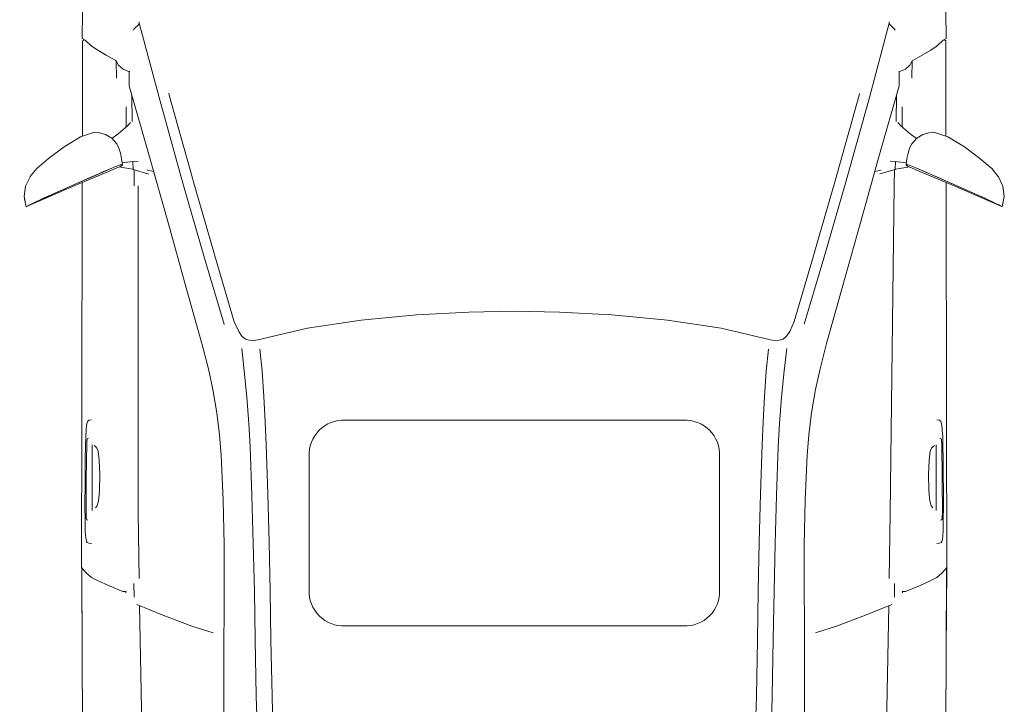
# Model space of a CAD drawing. Units: millimetres. Extents: x 595116 to 630915, y 909473 to 920225.
# Tile 116 of 134: x 629331 to 629397, y 919466 to 919512. Entities that reach past the tile are written whole.
import ezdxf

# ---------------------------------------------------------------- set-up
doc = ezdxf.new("R2010")
doc.units = ezdxf.units.MM
doc.layers.add('C-PRKG-VEHI', color=8, linetype='Continuous', lineweight=13)
doc.layers.add('Dimension', color=3, linetype='Continuous', lineweight=18)
doc.styles.get("Standard").update_dxf_attribs({"font": 'arial.ttf'})
doc.dimstyles.new('ISO-25', dxfattribs={"dimtxt": 9, "dimasz": 6, "dimexe": 1.25, "dimexo": 0.625, "dimtad": 1, "dimlunit": 4, "dimtxsty": 'Standard', "dimcen": 2.5, "dimadec": 0, "dimazin": 0, "dimtfac": 1, "dimtmove": 0, "dimatfit": 3, "dimfxl": 1, "dimarcsym": 0})

# ---------------------------------------------------------------- blocks, each defined once
blk = doc.blocks.new('A$C7ADB3080')
for p, q in [((1725, 1949.3), (1706, 1940.5)), ((1745.5, 1952.4), (1725, 1949.3)), ((1765.9, 1948), (1745.5, 1952.4)), ((1765.8, 1948.2), (1752, 1951)), ((1765.7, 1947.4), (1752.8, 1918.2)), ((1763.8, 1944.5), (1759.4, 1935.8)), ((1762, 1941.3), (1763.8, 1944.5)), ((1763.8, 1944.5), (1765, 1946.2)), ((1765, 1946.2), (1765.7, 1947.4)), ((1765.7, 1947.4), (1765.9, 1948)), ((1765.9, 1948), (1765.8, 1948.2)), ((1689.8, 1927.3), (1669.6, 1903.9)), ((1705.6, 1940.3), (1689.8, 1927.3)), ((1706, 1940.5), (1705.6, 1940.3)), ((1752.5, 1921.9), (1756.2, 1929.1)), ((1756.2, 1929.1), (1759.4, 1935.8)), ((1759.4, 1935.8), (1762, 1941.3)), ((1759.4, 1935.8), (1759.4, 1935.8)), ((1669.6, 1903.9), (1646.3, 1872.8)), ((1724.2, 1852.4), (1752.8, 1918.2)), ((1734, 1880.4), (1744, 1903.1)), ((1749.1, 1914.3), (1742, 1898.2)), ((1744, 1903.1), (1746, 1907.5)), ((1746, 1907.5), (1748.3, 1912.5)), ((1748.3, 1912.5), (1750.6, 1917.5)), ((1750.6, 1917.5), (1752.5, 1921.9)), ((1752.5, 1921.9), (1752.5, 1921.9)), ((1742, 1898.2), (1723, 1855.1)), ((1646.3, 1872.8), (1626.7, 1840.1)), ((1721.5, 1852), (1734, 1880.4)), ((1724.2, 1852.4), (1697.4, 1788.7)), ((1723, 1855.1), (1704.1, 1812.4)), ((1709.1, 1823.9), (1721.5, 1852)), ((1377.3, 1836), (1430.5, 1836.5)), ((1434.1, 1830.8), (1430.5, 1836.5)), ((1433.4, 1831.8), (1433.4, 1833.5)), ((1433.4, 1833.5), (1433.5, 1833.5)), ((1433.5, 1833.5), (1433.6, 1833.6)), ((1435.6, 1835.7), (1433.6, 1833.6)), ((1445.2, 1818.8), (1434.1, 1830.8)), ((1435.6, 1835.7), (1437, 1835.7)), ((1437, 1835.7), (1625.4, 1836.2)), ((1626.7, 1840.1), (1617.6, 1812)), ((1717.5, 1836.5), (2187.9, 1837.4)), ((2187.9, 1837.4), (2484.5, 1837.8)), ((2193.4, 1826), (2191.2, 1823.4)), ((2200.6, 1827.9), (2193.4, 1826)), ((2210.5, 1828.9), (2200.6, 1827.9)), ((2224.9, 1829.7), (2210.5, 1828.9)), ((2224.9, 1829.7), (2241, 1830)), ((2227.3, 1826.2), (2226.9, 1824.2)), ((2227.3, 1826.2), (2228.5, 1826.8)), ((2229.6, 1827.1), (2228.5, 1826.8)), ((2232.9, 1827.6), (2229.6, 1827.1)), ((2237.6, 1827.8), (2232.9, 1827.6)), ((2309.4, 1828.6), (2237.6, 1827.8)), ((2241, 1830), (2270.8, 1830.6)), ((2270.8, 1830.6), (2301.2, 1830.8)), ((2301.2, 1830.8), (2330.4, 1831.1)), ((2377.2, 1829.1), (2309.4, 1828.6)), ((2330.4, 1831.1), (2346.2, 1831.1)), ((2346.2, 1831.1), (2361.6, 1831.1)), ((2361.6, 1831.1), (2390.1, 1830.9)), ((2382.2, 1828.9), (2377.2, 1829.1)), ((2386.2, 1828.5), (2382.2, 1828.9)), ((2388.4, 1827.8), (2386.2, 1828.5)), ((2386.8, 1828.4), (2387.6, 1828.3)), ((2387.6, 1828.3), (2389.6, 1827.5)), ((2389.6, 1827.5), (2388.4, 1827.8)), ((2389.6, 1827.5), (2389.9, 1825.3)), ((2411.1, 1830.5), (2390.1, 1830.9)), ((2420.6, 1830), (2411.1, 1830.5)), ((2428.8, 1829.1), (2420.6, 1830)), ((2432.5, 1828.1), (2428.8, 1829.1)), ((2434.5, 1826.7), (2432.5, 1828.1)), ((2435.7, 1823.3), (2434.5, 1826.7)), ((2494.5, 1829.3), (2484.5, 1837.8)), ((2484.8, 1837.6), (2652.6, 1836.8)), ((2485.1, 1837.3), (2485.3, 1837.5)), ((2485.3, 1837.5), (2485.4, 1837.5)), ((2654.1, 1836.7), (2485.4, 1837.5)), ((2496.6, 1827.5), (2494.5, 1829.3)), ((2503.9, 1818.7), (2496.6, 1827.5)), ((2652.6, 1836.8), (2920.1, 1835.4)), ((2925, 1835.1), (2654.1, 1836.7)), ((1445.7, 1818.2), (1445.2, 1818.8)), ((1446.6, 1816.9), (1445.7, 1818.2)), ((1453.9, 1805.9), (1446.6, 1816.9)), ((1464, 1789.1), (1453.9, 1805.9)), ((1617.6, 1812), (1618.4, 1802.1)), ((1704.1, 1812.4), (1694.1, 1789.9)), ((1699.6, 1802.3), (1709.1, 1823.9)), ((2190.4, 1818.3), (2191.2, 1823.4)), ((2240, 1816.8), (2309.6, 1816.6)), ((2243.3, 1810.5), (2241.1, 1813.1)), ((2246.7, 1807.3), (2243.3, 1810.5)), ((2252.5, 1804.7), (2246.7, 1807.3)), ((2270.3, 1802.6), (2252.5, 1804.7)), ((2309.6, 1816.6), (2370.7, 1816.9)), ((2354, 1805), (2346.9, 1803.3)), ((2361.4, 1807), (2354, 1805)), ((2365.7, 1810.3), (2361.4, 1807)), ((2436.2, 1818.2), (2435.7, 1823.3)), ((2504.3, 1818.2), (2503.9, 1818.7)), ((2505, 1816.9), (2504.3, 1818.2)), ((2510.7, 1805), (2505, 1816.9)), ((2520.5, 1784.5), (2510.7, 1805)), ((1474.9, 1770), (1464, 1789.1)), ((1618.4, 1802.1), (1622.1, 1790.1)), ((1622.1, 1790.1), (1629.3, 1778)), ((1697.4, 1788.7), (1685.2, 1759.7)), ((1694.1, 1789.9), (1688.5, 1776.5)), ((1691.4, 1783.7), (1694.6, 1791)), ((1691.4, 1783.7), (1694.1, 1789.9)), ((1694.1, 1789.9), (1694.6, 1791)), ((1694.6, 1791), (1695.1, 1792.1)), ((1695.1, 1792.1), (1695.6, 1793.4)), ((1695.6, 1793.4), (1696.2, 1794.5)), ((1696.2, 1794.5), (1697.1, 1796.7)), ((1697.1, 1796.7), (1698.1, 1798.8)), ((1698.1, 1798.8), (1698.9, 1800.7)), ((1698.9, 1800.7), (1699.6, 1802.3)), ((2299.3, 1801.5), (2270.3, 1802.6)), ((2330.4, 1802), (2299.3, 1801.5)), ((2346.9, 1803.3), (2330.4, 1802)), ((1475.5, 1768.9), (1474.9, 1770)), ((1510, 1768.4), (1475.5, 1768.9)), ((1476.3, 1768.3), (1475.5, 1768.9)), ((1483.6, 1764.1), (1476.3, 1768.3)), ((1629.8, 1777.6), (1620.9, 1764.8)), ((1629.3, 1778), (1640.8, 1767.9)), ((1640.8, 1767.9), (1649.1, 1763.8)), ((1688.5, 1776.5), (1683.2, 1763.2)), ((1683.2, 1763.2), (1685.6, 1769.3)), ((1685.6, 1769.3), (1688.5, 1776.5)), ((1688.5, 1776.5), (1691.4, 1783.7)), ((2532.1, 1755.6), (2520.5, 1784.5)), ((1491.8, 1755.3), (1483.6, 1764.1)), ((1496.1, 1745.8), (1491.8, 1755.3)), ((1496.8, 1742), (1496.1, 1745.8)), ((1607.1, 1748.9), (1567, 1748.9)), ((1604.9, 1746.4), (1597.9, 1740.6)), ((1620.9, 1764.8), (1604.9, 1746.4)), ((1649.1, 1763.8), (1658.9, 1760.6)), ((1658.9, 1760.6), (1670.1, 1758.3)), ((1670.1, 1758.3), (1682.7, 1756.6)), ((1675.9, 1734.9), (1677.6, 1752)), ((1677.6, 1752), (1678.3, 1757.2)), ((1683.2, 1763.2), (1682.2, 1758.7)), ((1682.2, 1758.7), (1682.5, 1760.9)), ((1682.3, 1757.1), (1682.2, 1758.7)), ((1682.2, 1758.7), (1682.7, 1756.6)), ((1682.7, 1756.6), (1682.3, 1757.1)), ((1682.5, 1760.9), (1683.2, 1763.2)), ((1682.7, 1756.6), (1684, 1757.5)), ((1683.3, 1756.9), (1682.7, 1756.6)), ((1684, 1757.5), (1683.3, 1756.9)), ((1684, 1757.5), (1685.2, 1759.7)), ((1684.6, 1758.5), (1684, 1757.5)), ((1685.2, 1759.7), (1684.6, 1758.5)), ((1688, 1756.4), (1686.5, 1762.7)), ((1690, 1743.9), (1688, 1756.4)), ((2532.1, 1755.6), (2532.1, 1749.2)), ((2533.9, 1749.8), (2532.1, 1749.8)), ((2534.6, 1749.8), (2533.9, 1749.8)), ((1411.9, 1733.6), (1401.3, 1722.8)), ((1414.5, 1734.8), (1411.9, 1733.6)), ((1524.8, 1743.1), (1496.6, 1743.1)), ((1661.6, 1703.9), (1524.8, 1743.1)), ((1596, 1736.9), (1543.4, 1737.8)), ((1675.3, 1725.1), (1675.9, 1734.9)), ((1692, 1735.3), (1676, 1735.6)), ((1690.8, 1736.6), (1690, 1743.9)), ((1690.9, 1735.3), (1690.8, 1736.6)), ((1700.5, 1704.4), (1692, 1735.3)), ((1724.4, 1733.1), (1692.5, 1733.5)), ((2375.6, 1724.9), (1724.4, 1733.1)), ((2543.4, 1733.4), (2516.3, 1733.9)), ((2579.5, 1676.2), (2558, 1728.1)), ((1397.7, 1723.7), (1548.1, 1683.7)), ((1692.9, 1707.2), (1693, 1706.9)), ((1693, 1706.9), (1695.6, 1694.4)), ((2506, 1723.1), (2375.6, 1724.9)), ((2594.2, 1721.7), (2560.4, 1722.3)), ((3148.3, 1710.7), (2594.2, 1721.7)), ((1799.6, 1665.1), (1661.6, 1703.9)), ((1548.1, 1683.7), (1718.6, 1636)), ((2601.1, 1618), (2579.5, 1676.2)), ((1543.7, 1663.2), (1540.2, 1664.1)), ((1714, 1615.6), (1543.7, 1663.2)), ((1927.3, 1629.4), (1799.6, 1665.1)), ((1718.6, 1636), (1868.2, 1592.8)), ((2038.3, 1598.2), (1927.3, 1629.4)), ((1714, 1615.6), (1708.7, 1617.1)), ((1860.7, 1573.2), (1714, 1615.6)), ((2614.2, 1576.1), (2601.1, 1618)), ((1868.2, 1592.8), (2000, 1553.9)), ((2088.8, 1585.4), (2038.3, 1598.2)), ((1863.6, 1572.4), (1860.7, 1573.2)), ((1994.6, 1533.7), (1863.6, 1572.4)), ((2130.1, 1576.2), (2088.8, 1585.4)), ((2176.5, 1568.6), (2130.1, 1576.2)), ((2220.1, 1563.2), (2176.5, 1568.6)), ((2260.3, 1559.8), (2220.1, 1563.2)), ((2350.4, 1555.7), (2260.3, 1559.8)), ((2439.2, 1554), (2350.4, 1555.7)), ((2529.7, 1553.9), (2439.2, 1554)), ((2589.2, 1554.1), (2529.7, 1553.9)), ((2589.2, 1554.1), (2618.6, 1554.3)), ((2589.2, 1554.1), (2589.2, 1554.1)), ((2622.6, 1554.3), (2618.6, 1554.3)), ((2773, 1554.3), (2622.6, 1554.3)), ((2014.5, 1525), (1992.9, 1534.5)), ((2023.9, 1518.6), (2014.5, 1525)), ((2029.9, 1511.6), (2023.9, 1518.6)), ((2031.7, 1503.8), (2029.9, 1511.6)), ((2092.8, 1514), (2048.5, 1519)), ((2048.5, 1519), (2092.8, 1514)), ((2145.3, 1508.8), (2092.8, 1514)), ((2092.8, 1514), (2145.3, 1508.8)), ((2030.9, 1486.7), (2032.1, 1494.6)), ((2032.1, 1494.6), (2031.7, 1503.8)), ((2197.8, 1504.5), (2145.3, 1508.8)), ((2145.3, 1508.8), (2197.8, 1504.5)), ((2244.2, 1501.9), (2197.8, 1504.5)), ((2197.8, 1504.5), (2244.2, 1501.9)), ((2341, 1498.7), (2244.2, 1501.9)), ((2244.2, 1501.9), (2341, 1498.7)), ((2436.5, 1496), (2341, 1498.7)), ((2341, 1498.7), (2436.5, 1496)), ((2531.6, 1493.8), (2436.5, 1496)), ((2436.5, 1496), (2531.6, 1493.8)), ((2627.7, 1492.2), (2531.6, 1493.8)), ((2531.6, 1493.8), (2627.7, 1492.2)), ((2739.8, 1490), (2627.7, 1492.2)), ((2627.7, 1492.2), (2739.8, 1490)), ((2007.4, 1388.1), (2030.9, 1486.7)), ((2049.5, 1482.6), (2093, 1478.3)), ((2093, 1478.3), (2049.5, 1482.6)), ((2093, 1478.3), (2143.5, 1474.7)), ((2143.5, 1474.7), (2093, 1478.3)), ((2143.5, 1474.7), (2194, 1471.9)), ((2194, 1471.9), (2143.5, 1474.7)), ((2194, 1471.9), (2239.7, 1470.1)), ((2239.7, 1470.1), (2194, 1471.9)), ((2855.6, 1486.9), (2739.8, 1490)), ((2739.8, 1490), (2855.6, 1486.9)), ((2239.7, 1470.1), (2337.4, 1467)), ((2337.4, 1467), (2239.7, 1470.1)), ((2337.4, 1467), (2434.6, 1464.3)), ((2434.6, 1464.3), (2337.4, 1467)), ((2434.6, 1464.3), (2531.7, 1462.2)), ((2531.7, 1462.2), (2434.6, 1464.3)), ((2531.7, 1462.2), (2628.6, 1460.7)), ((2628.6, 1460.6), (2531.7, 1462.2)), ((2628.6, 1460.7), (2740.5, 1458.5)), ((2740.5, 1458.5), (2628.6, 1460.6)), ((2628.8, 1460.7), (2628.8, 1460.6)), ((2740.5, 1458.5), (2856, 1455.4)), ((2856, 1455.4), (2740.5, 1458.5)), ((1991.5, 1281.2), (2007.4, 1388.1)), ((2263, 1385.3), (2528.8, 1385.3)), ((2395.9, 1385.3), (2466.3, 1385.3)), ((2191, 1313.5), (2191, 639.5)), ((2600.7, 1313.5), (2600.7, 639.5)), ((1981.3, 1170.9), (1991.5, 1281.2)), ((1976, 1066.4), (1981.3, 1170.9)), ((1974.1, 976.2), (1976, 1066.4)), ((1976, 886), (1974.1, 976.2)), ((1981.3, 781.5), (1976, 886)), ((1991.5, 671.2), (1981.3, 781.5)), ((2007.4, 564.3), (1991.5, 671.2)), ((2030.9, 465.7), (2007.4, 564.3)), ((2263, 567.7), (2528.8, 567.7)), ((2628.6, 491.7), (2531.7, 490.1)), ((2531.7, 490.1), (2628.6, 491.7)), ((2740.5, 493.9), (2628.6, 491.7)), ((2628.6, 491.7), (2740.5, 493.9)), ((2856, 496.9), (2740.5, 493.9)), ((2740.5, 493.9), (2856, 496.9)), ((2093, 474.1), (2049.5, 469.8)), ((2049.5, 469.8), (2093, 474.1)), ((2143.5, 477.7), (2093, 474.1)), ((2093, 474.1), (2143.5, 477.7)), ((2194, 480.4), (2143.5, 477.7)), ((2143.5, 477.7), (2194, 480.4)), ((2239.7, 482.3), (2194, 480.4)), ((2194, 480.4), (2239.7, 482.3)), ((2337.4, 485.4), (2239.7, 482.3)), ((2239.7, 482.3), (2337.4, 485.4)), ((2434.6, 488), (2337.4, 485.4)), ((2337.4, 485.4), (2434.6, 488)), ((2531.7, 490.1), (2434.6, 488)), ((2434.6, 488), (2531.7, 490.1)), ((2032.1, 457.8), (2030.9, 465.7)), ((2031.7, 448.5), (2032.1, 457.8)), ((2244.2, 450.5), (2341, 453.7)), ((2341, 453.7), (2244.2, 450.5)), ((2341, 453.7), (2436.5, 456.4)), ((2436.5, 456.4), (2341, 453.7)), ((2436.5, 456.4), (2531.6, 458.6)), ((2531.6, 458.6), (2436.5, 456.4)), ((2531.6, 458.6), (2627.7, 460.2)), ((2627.7, 460.2), (2531.6, 458.6)), ((2627.7, 460.2), (2739.8, 462.4)), ((2739.8, 462.4), (2627.7, 460.2)), ((2739.8, 462.4), (2855.6, 465.5)), ((2855.6, 465.5), (2739.8, 462.4)), ((2014.5, 427.4), (2023.9, 433.8)), ((2023.9, 433.8), (2029.9, 440.8)), ((2029.9, 440.8), (2031.7, 448.5)), ((2048.5, 433.4), (2092.8, 438.4)), ((2092.8, 438.4), (2048.5, 433.4)), ((2092.8, 438.4), (2145.3, 443.6)), ((2145.3, 443.6), (2092.8, 438.4)), ((2145.3, 443.6), (2197.8, 447.9)), ((2197.8, 447.9), (2145.3, 443.6)), ((2197.8, 447.9), (2244.2, 450.5)), ((2244.2, 450.5), (2197.8, 447.9)), ((1863.6, 380), (1994.8, 418.7)), ((1994.8, 418.7), (2014.5, 427.4)), ((2000, 398.5), (1868.2, 359.6)), ((2000, 398.5), (2000.4, 398.7)), ((2220.1, 389.2), (2260.3, 392.6)), ((2260.3, 392.6), (2350.4, 396.7)), ((2350.4, 396.7), (2439.2, 398.4)), ((2439.2, 398.4), (2529.7, 398.5)), ((2529.7, 398.5), (2589.2, 398.2)), ((2589.2, 398.2), (2589.2, 398.3)), ((2618.6, 398.1), (2589.2, 398.2)), ((2618.6, 398.1), (2622.6, 398.1)), ((2622.6, 398.1), (2773, 398.1)), ((1714, 336.8), (1860.7, 379.1)), ((1860.7, 379.1), (1863.6, 380)), ((2088.8, 367), (2130.1, 376.2)), ((2130.1, 376.2), (2176.5, 383.8)), ((2176.5, 383.8), (2220.1, 389.2)), ((2601.1, 334.3), (2614.2, 376.3)), ((1868.2, 359.6), (1718.6, 316.3)), ((1927.3, 323), (2038.3, 354.2)), ((2038.3, 354.2), (2088.8, 367)), ((1543.7, 289.1), (1708.7, 335.3)), ((1708.7, 335.3), (1714, 336.8)), ((2579.5, 276.2), (2601.1, 334.3)), ((1718.6, 316.3), (1548.1, 268.7)), ((1799.6, 287.3), (1927.3, 323)), ((1539.5, 288), (1543.7, 289.1)), ((1661.6, 248.5), (1799.6, 287.3)), ((2558, 224.3), (2579.5, 276.2)), ((1548.1, 268.7), (1397.7, 228.7)), ((1695.6, 258), (1693, 245.5)), ((1524.8, 209.3), (1661.6, 248.5)), ((1692, 217.1), (1700.7, 248.5)), ((1693, 245.5), (1692.9, 245.3)), ((2594.2, 230.7), (3148.3, 241.7)), ((1401.3, 229.6), (1411.9, 218.7)), ((1411.9, 218.7), (1414.5, 217.6)), ((1675.9, 217.5), (1675.3, 227.3)), ((1677.6, 200.4), (1675.9, 217.5)), ((1676, 216.8), (1692, 217.1)), ((1690, 208.5), (1690.8, 215.8)), ((1690.8, 215.8), (1690.9, 217.1)), ((1692.5, 218.9), (1724.4, 219.2)), ((1724.4, 226.9), (2375.6, 227.4)), ((2375.6, 227.4), (2506, 229.2)), ((2516.3, 218.5), (2543.4, 219)), ((2560.4, 230.1), (2594.2, 230.7)), ((1483.6, 188.2), (1491.8, 197.1)), ((1491.8, 197.1), (1496.1, 206.6)), ((1496.1, 206.6), (1496.8, 210.3)), ((1496.6, 209.3), (1524.8, 209.3)), ((1543.4, 214.6), (1596, 215.5)), ((1566.6, 203.4), (1607.1, 203.4)), ((1598, 211.8), (1604.9, 206)), ((1604.9, 206), (1620.9, 187.6)), ((1678.3, 195.2), (1677.6, 200.4)), ((1688, 196), (1690, 208.5)), ((2520.5, 167.9), (2532.1, 196.8)), ((2532.1, 203.2), (2532.1, 196.8)), ((2532.1, 202.6), (2533.9, 202.6)), ((2533.9, 202.6), (2534.6, 202.6)), ((1464, 163.2), (1474.9, 182.4)), ((1474.9, 182.4), (1475.5, 183.5)), ((1475.5, 183.5), (1476.3, 184.1)), ((1475.5, 183.5), (1510, 183.9)), ((1476.3, 184.1), (1483.6, 188.2)), ((1620.9, 187.6), (1629.8, 174.8)), ((1640.8, 184.4), (1629.3, 174.4)), ((1649.1, 188.6), (1640.8, 184.4)), ((1658.9, 191.7), (1649.1, 188.6)), ((1670.1, 194.1), (1658.9, 191.7)), ((1682.7, 195.8), (1670.1, 194.1)), ((1682.7, 195.8), (1682.2, 193.7)), ((1682.2, 193.7), (1682.3, 195.3)), ((1682.5, 191.5), (1682.2, 193.7)), ((1682.2, 193.7), (1683.2, 189.1)), ((1682.3, 195.3), (1682.7, 195.8)), ((1683.2, 189.1), (1682.5, 191.5)), ((1682.7, 195.8), (1683.3, 195.5)), ((1684, 194.8), (1682.7, 195.8)), ((1685.6, 183), (1683.2, 189.1)), ((1683.2, 189.1), (1688.5, 175.8)), ((1683.3, 195.5), (1684, 194.8)), ((1684, 194.8), (1684.6, 193.9)), ((1685.2, 192.7), (1684, 194.8)), ((1684.6, 193.9), (1685.2, 192.7)), ((1685.2, 192.7), (1697.4, 163.7)), ((1688.5, 175.8), (1685.6, 183)), ((1686.5, 189.6), (1688, 196)), ((1453.9, 146.5), (1464, 163.2)), ((1622.1, 162.3), (1618.4, 150.3)), ((1629.3, 174.4), (1622.1, 162.3)), ((1691.4, 168.6), (1688.5, 175.8)), ((1688.5, 175.8), (1694.1, 162.5)), ((1694.6, 161.4), (1691.4, 168.6)), ((1694.1, 162.5), (1691.4, 168.6)), ((1694.6, 161.4), (1694.1, 162.5)), ((1694.1, 162.5), (1704.1, 140)), ((1695.1, 160.2), (1694.6, 161.4)), ((1695.6, 159), (1695.1, 160.2)), ((1696.2, 157.8), (1695.6, 159)), ((1697.1, 155.6), (1696.2, 157.8)), ((1697.4, 163.7), (1724.2, 100)), ((2510.7, 147.4), (2520.5, 167.9)), ((1446.6, 135.5), (1453.9, 146.5)), ((1618.4, 150.3), (1617.6, 140.4)), ((1617.6, 140.4), (1626.7, 112.3)), ((1698.1, 153.6), (1697.1, 155.6)), ((1698.9, 151.7), (1698.1, 153.6)), ((1699.6, 150.1), (1698.9, 151.7)), ((1709.1, 128.5), (1699.6, 150.1)), ((1704.1, 140), (1723, 97.3)), ((2241.1, 139.3), (2243.3, 141.9)), ((2243.3, 141.9), (2246.7, 145.1)), ((2246.7, 145.1), (2252.5, 147.6)), ((2252.5, 147.6), (2270.3, 149.7)), ((2270.3, 149.7), (2299.3, 150.8)), ((2299.3, 150.8), (2330.4, 150.4)), ((2330.4, 150.4), (2346.9, 149.1)), ((2346.9, 149.1), (2354, 147.3)), ((2354, 147.3), (2361.4, 145.4)), ((2361.4, 145.4), (2365.7, 142)), ((2505, 135.5), (2510.7, 147.4)), ((1430.5, 115.9), (1434.1, 121.6)), ((1433.4, 118.9), (1433.4, 120.5)), ((1433.5, 118.8), (1433.4, 118.9)), ((1433.6, 118.7), (1433.5, 118.8)), ((1433.6, 118.7), (1435.6, 116.7)), ((1434.1, 121.6), (1445.2, 133.5)), ((1445.2, 133.5), (1445.7, 134.2)), ((1445.7, 134.2), (1446.6, 135.5)), ((1721.5, 100.4), (1709.1, 128.5)), ((2191.2, 129), (2190.4, 134.1)), ((2191.2, 129), (2193.4, 126.4)), ((2193.4, 126.4), (2200.6, 124.5)), ((2200.6, 124.5), (2210.5, 123.4)), ((2210.5, 123.4), (2224.9, 122.7)), ((2241, 122.3), (2224.9, 122.7)), ((2226.9, 128.1), (2227.3, 126.2)), ((2228.5, 125.6), (2227.3, 126.2)), ((2228.5, 125.6), (2229.6, 125.3)), ((2229.6, 125.3), (2232.9, 124.8)), ((2232.9, 124.8), (2237.6, 124.6)), ((2237.6, 124.6), (2309.4, 123.8)), ((2309.6, 135.8), (2240, 135.5)), ((2270.8, 121.8), (2241, 122.3)), ((2301.2, 121.5), (2270.8, 121.8)), ((2330.4, 121.3), (2301.2, 121.5)), ((2309.4, 123.8), (2377.2, 123.3)), ((2370.7, 135.5), (2309.6, 135.8)), ((2346.2, 121.2), (2330.4, 121.3)), ((2361.6, 121.2), (2346.2, 121.2)), ((2390.1, 121.5), (2361.6, 121.2)), ((2377.2, 123.3), (2382.2, 123.4)), ((2382.2, 123.4), (2386.2, 123.8)), ((2386.2, 123.8), (2388.4, 124.5)), ((2387.6, 124.1), (2386.9, 124)), ((2389.6, 124.9), (2387.6, 124.1)), ((2388.4, 124.5), (2389.6, 124.9)), ((2389.9, 127.1), (2389.6, 124.9)), ((2390.1, 121.5), (2411.1, 121.9)), ((2411.1, 121.9), (2420.6, 122.4)), ((2420.6, 122.4), (2428.8, 123.3)), ((2428.8, 123.3), (2432.5, 124.2)), ((2432.5, 124.2), (2434.5, 125.7)), ((2434.5, 125.7), (2435.7, 129.1)), ((2435.7, 129.1), (2436.2, 134.1)), ((2484.5, 114.5), (2494.5, 123.1)), ((2494.5, 123.1), (2496.6, 124.8)), ((2496.6, 124.8), (2503.9, 133.7)), ((2503.9, 133.7), (2504.3, 134.2)), ((2504.3, 134.2), (2505, 135.5)), ((1430.5, 115.9), (1377.3, 116.3)), ((1437, 116.6), (1435.6, 116.7)), ((1625.4, 116.1), (1437, 116.6)), ((1626.7, 112.3), (1646.3, 79.6)), ((2187.9, 115), (1717.5, 115.9)), ((1734, 72), (1721.5, 100.4)), ((1752.8, 34.1), (1724.2, 100)), ((2484.5, 114.5), (2187.9, 115)), ((2485.3, 114.8), (2484.9, 114.8)), ((2485.3, 114.8), (2485.1, 115)), ((2485.4, 114.8), (2485.3, 114.8)), ((2485.4, 114.8), (2654.1, 115.7)), ((2652.6, 115.6), (2496.9, 114.9)), ((2920.1, 117), (2652.6, 115.6)), ((2924.7, 117.2), (2654.1, 115.7)), ((1646.3, 79.6), (1669.6, 48.5)), ((1723, 97.3), (1742, 54.2)), ((1744, 49.2), (1734, 72)), ((1669.6, 48.5), (1689.8, 25)), ((1742, 54.2), (1749.2, 38)), ((1746, 44.9), (1744, 49.2)), ((1748.3, 39.9), (1746, 44.9)), ((1750.6, 34.9), (1748.3, 39.9)), ((1689.8, 25), (1705.6, 12.1)), ((1752.5, 30.5), (1750.6, 34.9)), ((1756.2, 23.3), (1752.5, 30.5)), ((1752.5, 30.5), (1752.5, 30.5)), ((1752.8, 34.1), (1765.7, 5)), ((1759.4, 16.5), (1756.2, 23.3)), ((1705.6, 12.1), (1706, 11.9)), ((1706, 11.9), (1725, 3)), ((1725, 3), (1745.5, 0)), ((1745.5, 0), (1765.9, 4.4)), ((1749.9, 0.9), (1765.8, 4.2)), ((1759.4, 16.6), (1759.4, 16.5)), ((1762, 11.1), (1759.4, 16.5)), ((1759.4, 16.5), (1763.8, 7.9)), ((1763.8, 7.9), (1762, 11.1)), ((1765, 6.2), (1763.8, 7.9)), ((1765.7, 5), (1765, 6.2)), ((1765.9, 4.4), (1765.7, 5)), ((1765.8, 4.2), (1765.9, 4.4))]:
    blk.add_line(p, q)
for centre, start, end in [((2259.6, 1316.8), 87.1848, 182.6876), ((2532.2, 1316.8), 357.3124, 92.8152), ((2259.6, 636.3), 177.3124, 272.8152), ((2532.2, 636.3), 267.1848, 2.6876)]:
    blk.add_arc(centre, 68.6, start, end)
blk = doc.blocks.new('*D152')
at = {"layer": 'Defpoints', "color": 0, "transparency": 16777216}
for p in [(629325.041, 919429.828), (629327.741, 919429.828), (629325.041, 919411.828)]:
    blk.add_point(p, dxfattribs=at)
at = {"layer": 'Dimension', "color": 0, "lineweight": -2, "transparency": 16777216}
for p, q in [((629327.741, 919429.828), (629327.741, 919524.671)), ((629325.666, 919429.828), (629328.991, 919429.828)), ((629327.741, 919417.828), (629327.741, 919423.828)), ((629325.666, 919411.828), (629328.991, 919411.828))]:
    blk.add_line(p, q, dxfattribs=at)
at = {"layer": 'Dimension', "color": 0, "transparency": 16777216}
for points in [[(629326.741, 919423.828), (629328.741, 919423.828), (629327.741, 919429.828)], [(629326.741, 919417.828), (629328.741, 919417.828), (629327.741, 919411.828)]]:
    blk.add_solid(points, dxfattribs=at)
at = {"layer": 'Dimension', "color": 0, "transparency": 16777216, "insert": (629322.459, 919480.25), "char_height": 9, "attachment_point": 5, "rotation": 90}
blk.add_mtext('COL. 1\'-6" TYP.', dxfattribs=at)

msp = doc.modelspace()

# ---------------------------------------------------------------- block references
at = {"layer": 'C-PRKG-VEHI', "xscale": 0.0334614614063694, "yscale": 0.0334614614063694, "zscale": 0.0334614614063694, "rotation": 270}
msp.add_blockref('A$C7ADB3080', (629331.465, 919558.166), dxfattribs=at)

# ---------------------------------------------------------------- dimensions: what is measured, and where the dimension line sits
at = {"layer": 'Dimension'}
dim = msp.add_linear_dim(base=(629327.741, 919429.828), p1=(629325.041, 919411.828), p2=(629325.041, 919429.828), angle=90, text='COL. <> TYP.', dimstyle='ISO-25', override={"dimdec": 1, "dimlfac": 1, "dimrnd": 0, "dimzin": 1, "dimdsep": 46, "dimlunit": 4, "dimfrac": 2}, dxfattribs=at)
dim.commit()
dim.dimension.update_dxf_attribs({"geometry": '*D152', "text_midpoint": (629322.459, 919480.25)})

doc.saveas('drawing.dxf')
